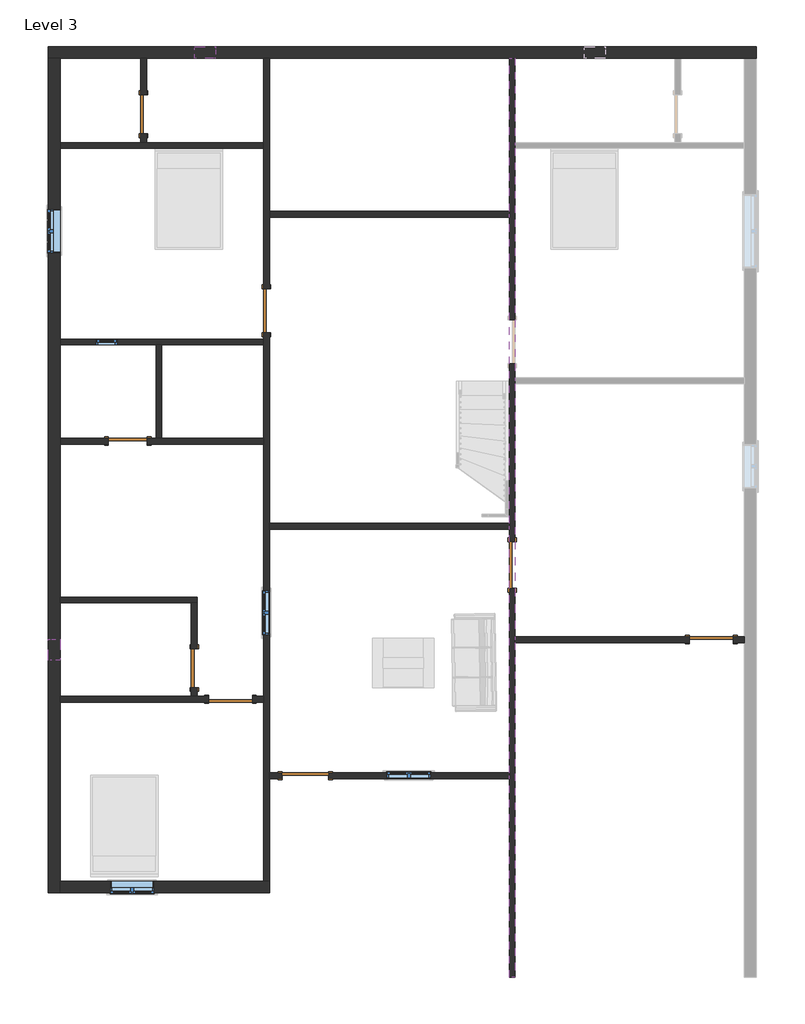
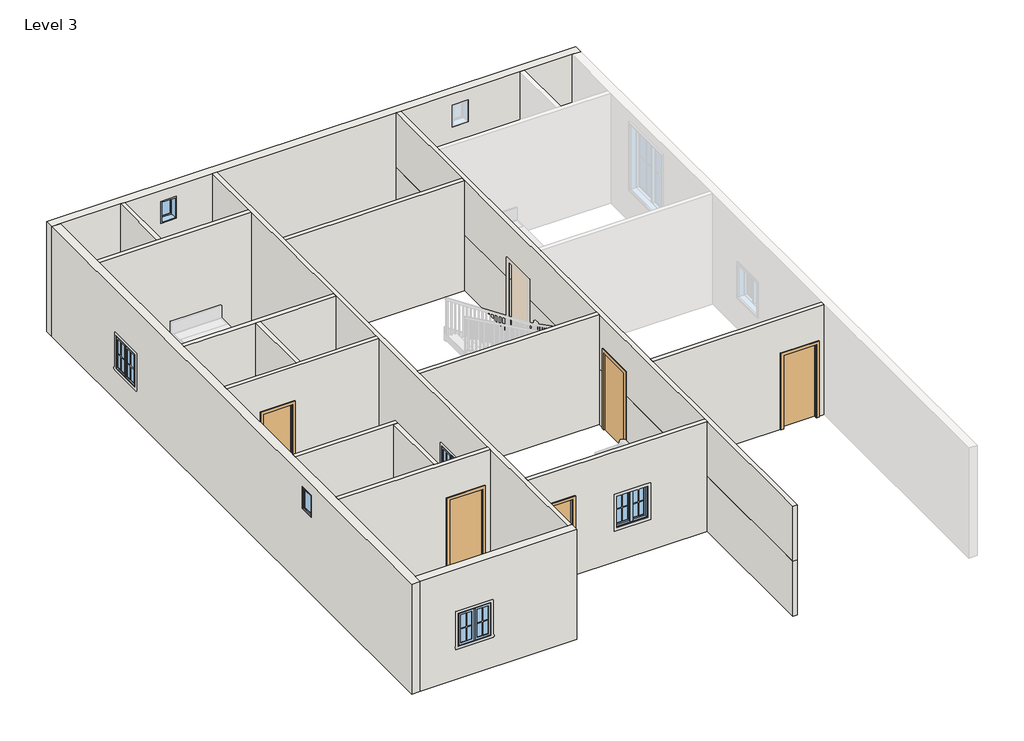
# One storey, part 1 of 3: 18 walls, 8 doors, 7 windows.
"""IFC4 building model written with IfcOpenShell, lengths in millimetres."""

from ifc_helpers import new_model, si_unit, frame, origin, place, context, project, spatial, polyline, outline, extrude, faceted_brep, transform, mapped, element, save
from components import door_f2b275c1, door_d8f5dbb5, door_825b8444, door_c29894e6, door_305aa2a5, window_aa618e30, window_a10b4202, window_339605e1, window_a598f463

model = new_model("IFC4")

# Units and contexts
model_context = context("Model", 3, world=origin())
ifc_project = project(units=[si_unit("LENGTHUNIT", "METRE", prefix="MILLI")], contexts=[model_context])

# Site, building, storey
site = spatial("IfcSite", under=ifc_project)
building = spatial("IfcBuilding", under=site)
storey = spatial("IfcBuildingStorey", under=building, Name="Level 3", Elevation=3200.4)

# Doors
placement = place(None, origin())
door_shape = door_f2b275c1(model_context)
element("IfcDoor", 1, ObjectType="Single-Flush : 30\" x 80\"", at=placement, inside=storey, context=model_context, shape_type="MappedRepresentation", body=[
    mapped(door_shape, transform((-5639.8561469, 9100.7522623, 3200.4), x_axis=(0.0, -1.0, 0.0), y_axis=(1.0, 0.0, 0.0), z_axis=(0.0, 0.0, 1.0))),
])
element("IfcDoor", 2, ObjectType="Single-Flush : 30\" x 80\"", at=placement, inside=storey, context=model_context, shape_type="MappedRepresentation", body=[
    mapped(door_shape, transform((-4646.033646, -1745.0477377, 3200.4), x_axis=(0.0, -1.0, 0.0), y_axis=(1.0, 0.0, 0.0), z_axis=(0.0, 0.0, 1.0))),
])
door_2_shape = door_d8f5dbb5(model_context)
element("IfcDoor", 3, ObjectType="Single-Flush : 30\" x 80\"", at=placement, inside=storey, context=model_context, shape_type="MappedRepresentation", body=[
    mapped(door_2_shape, transform((-5947.8915084, 2699.9522623, 3200.4), x_axis=(1.0, 0.0, 0.0), y_axis=(0.0, 1.0, 0.0), z_axis=(0.0, 0.0, 1.0))),
])
door_3_shape = door_825b8444(model_context)
element("IfcDoor", 4, ObjectType="Single-Flush : 34\" x 80\"", at=placement, inside=storey, context=model_context, shape_type="MappedRepresentation", body=[
    mapped(door_3_shape, transform((-3230.0915084, 5252.6522623, 3200.4), x_axis=(0.0, -1.0, 0.0), y_axis=(1.0, 0.0, 0.0), z_axis=(0.0, 0.0, 1.0))),
])
element("IfcDoor", 5, ObjectType="Single-Flush : 34\" x 80\"", at=placement, inside=storey, context=model_context, shape_type="MappedRepresentation", body=[
    mapped(door_3_shape, transform((-3938.0625772, -2354.6477377, 3200.4), x_axis=(1.0, 0.0, 0.0), y_axis=(0.0, 1.0, 0.0), z_axis=(0.0, 0.0, 1.0))),
])
door_4_shape = door_c29894e6(model_context)
element("IfcDoor", 6, ObjectType="Single-Flush : 34\" x 80\"", at=placement, inside=storey, context=model_context, shape_type="MappedRepresentation", body=[
    mapped(door_4_shape, transform((5488.4584916, -1186.2477377, 3200.4), x_axis=(1.0, 0.0, 0.0), y_axis=(0.0, 1.0, 0.0), z_axis=(0.0, 0.0, 1.0))),
])
door_5_shape = door_305aa2a5(model_context)
element("IfcDoor", 7, ObjectType="Single-Flush : 36\" x 84\"", at=placement, inside=storey, context=model_context, shape_type="MappedRepresentation", body=[
    mapped(door_5_shape, transform((1583.2084916, 274.2522623, 3200.4), x_axis=(0.0, -1.0, 0.0), y_axis=(1.0, 0.0, 0.0), z_axis=(0.0, 0.0, 1.0))),
])
element("IfcDoor", 8, ObjectType="Single-Flush : 36\" x 84\"", at=placement, inside=storey, context=model_context, shape_type="MappedRepresentation", body=[
    mapped(door_5_shape, transform((-2468.0915084, -3853.2477377, 3200.4), x_axis=(-1.0, 0.0, 0.0), y_axis=(0.0, -1.0, 0.0), z_axis=(0.0, 0.0, 1.0))),
])

# Walls
element("IfcWall", 9, ObjectType="9\"", at=placement, inside=storey, context=model_context, shape_type="Brep", body=[
    faceted_brep([(-7503.6415084, 10199.3022623, 3200.4), (-7275.0415084, 10199.3022623, 3200.4), (-5697.0061469, 10199.3022623, 3200.4), (-5582.7061469, 10199.3022623, 3200.4), (-3287.2415084, 10199.3022623, 3200.4), (-3172.9415084, 10199.3022623, 3200.4), (1526.0584916, 10199.3022623, 3200.4), (1640.3584916, 10199.3022623, 3200.4), (4770.1866507, 10199.3022623, 3200.4), (4884.4866507, 10199.3022623, 3200.4), (6136.1584916, 10199.3022623, 3200.4), (6364.7584916, 10199.3022623, 3200.4), (6364.7584916, 10199.3022623, 6248.4), (6136.1584916, 10199.3022623, 6248.4), (4884.4866507, 10199.3022623, 6248.4), (4770.1866507, 10199.3022623, 6248.4), (1640.3584916, 10199.3022623, 6248.4), (1526.0584916, 10199.3022623, 6248.4), (-3172.9415084, 10199.3022623, 6248.4), (-3287.2415084, 10199.3022623, 6248.4), (-5582.7061469, 10199.3022623, 6248.4), (-5697.0061469, 10199.3022623, 6248.4), (-7275.0415084, 10199.3022623, 6248.4), (-7503.6415084, 10199.3022623, 6248.4), (-4231.7738276, 10199.3022623, 5943.6), (-4231.7738276, 10199.3022623, 5334.0), (-4638.1738276, 10199.3022623, 5334.0), (-4638.1738276, 10199.3022623, 5943.6), (3408.4725711, 10199.3022623, 5943.6), (3408.4725711, 10199.3022623, 5334.0), (3002.0725711, 10199.3022623, 5334.0), (3002.0725711, 10199.3022623, 5943.6), (-7503.6415084, 10427.9022623, 3200.4), (-7503.6415084, 10427.9022623, 6248.4), (6364.7584916, 10427.9022623, 6248.4), (6364.7584916, 10427.9022623, 3200.4), (-4231.7738276, 10427.9022623, 5943.6), (-4638.1738276, 10427.9022623, 5943.6), (-4638.1738276, 10427.9022623, 5334.0), (-4231.7738276, 10427.9022623, 5334.0), (3408.4725711, 10427.9022623, 5943.6), (3002.0725711, 10427.9022623, 5943.6), (3002.0725711, 10427.9022623, 5334.0), (3408.4725711, 10427.9022623, 5334.0)], [[[0, 1, 2, 3, 4, 5, 6, 7, 8, 9, 10, 11, 12, 13, 14, 15, 16, 17, 18, 19, 20, 21, 22, 23], [24, 25, 26, 27], [28, 29, 30, 31]], [[32, 33, 34, 35], [36, 37, 38, 39], [40, 41, 42, 43]], [[11, 10, 9, 8, 7, 6, 5, 4, 3, 2, 1, 0, 32, 35]], [[0, 23, 33, 32]], [[12, 11, 35, 34]], [[25, 24, 36, 39]], [[26, 25, 39, 38]], [[27, 26, 38, 37]], [[24, 27, 37, 36]], [[29, 28, 40, 43]], [[30, 29, 43, 42]], [[31, 30, 42, 41]], [[28, 31, 41, 40]], [[23, 22, 21, 20, 19, 18, 17, 16, 15, 14, 13, 12, 34, 33]]]),
])
element("IfcWall", 10, ObjectType="9\"", at=placement, inside=storey, context=model_context, shape_type="Brep", body=[
    faceted_brep([(-7503.6415084, 10199.3022623, 3200.4), (-7503.6415084, -6145.5977377, 3200.4), (-7503.6415084, -6145.5977377, 6248.4), (-7503.6415084, 10199.3022623, 6248.4), (-7503.6415084, -1179.8977377, 5943.6), (-7503.6415084, -1586.2977377, 5943.6), (-7503.6415084, -1586.2977377, 5334.0), (-7503.6415084, -1179.8977377, 5334.0), (-7503.6415084, 7246.5522623, 5029.2), (-7503.6415084, 6382.9522623, 5029.2), (-7503.6415084, 6382.9522623, 4114.8), (-7503.6415084, 7246.5522623, 4114.8), (-7275.0415084, 10199.3022623, 3200.4), (-7275.0415084, 10199.3022623, 6248.4), (-7275.0415084, 8548.3022623, 6248.4), (-7275.0415084, 8434.0022623, 6248.4), (-7275.0415084, 4700.2022623, 6248.4), (-7275.0415084, 4585.9022623, 6248.4), (-7275.0415084, 2757.1022623, 6248.4), (-7275.0415084, 2642.8022623, 6248.4), (-7275.0415084, -354.3977377, 6248.4), (-7275.0415084, -468.6977377, 6248.4), (-7275.0415084, -2297.4977377, 6248.4), (-7275.0415084, -2411.7977377, 6248.4), (-7275.0415084, -5916.9977377, 6248.4), (-7275.0415084, -6145.5977377, 6248.4), (-7275.0415084, -6145.5977377, 3200.4), (-7275.0415084, -5916.9977377, 3200.4), (-7275.0415084, -2411.7977377, 3200.4), (-7275.0415084, -2297.4977377, 3200.4), (-7275.0415084, -468.6977377, 3200.4), (-7275.0415084, -354.3977377, 3200.4), (-7275.0415084, 2642.8022623, 3200.4), (-7275.0415084, 2757.1022623, 3200.4), (-7275.0415084, 4585.9022623, 3200.4), (-7275.0415084, 4700.2022623, 3200.4), (-7275.0415084, 8434.0022623, 3200.4), (-7275.0415084, 8548.3022623, 3200.4), (-7275.0415084, -1179.8977377, 5943.6), (-7275.0415084, -1179.8977377, 5334.0), (-7275.0415084, -1586.2977377, 5334.0), (-7275.0415084, -1586.2977377, 5943.6), (-7275.0415084, 7246.5522623, 5029.2), (-7275.0415084, 7246.5522623, 4114.8), (-7275.0415084, 6382.9522623, 4114.8), (-7275.0415084, 6382.9522623, 5029.2)], [[[0, 1, 2, 3], [4, 5, 6, 7], [8, 9, 10, 11]], [[12, 13, 14, 15, 16, 17, 18, 19, 20, 21, 22, 23, 24, 25, 26, 27, 28, 29, 30, 31, 32, 33, 34, 35, 36, 37], [38, 39, 40, 41], [42, 43, 44, 45]], [[1, 0, 12, 37, 36, 35, 34, 33, 32, 31, 30, 29, 28, 27, 26]], [[0, 3, 13, 12]], [[2, 1, 26, 25]], [[39, 38, 4, 7]], [[40, 39, 7, 6]], [[41, 40, 6, 5]], [[38, 41, 5, 4]], [[43, 42, 8, 11]], [[44, 43, 11, 10]], [[45, 44, 10, 9]], [[42, 45, 9, 8]], [[3, 2, 25, 24, 23, 22, 21, 20, 19, 18, 17, 16, 15, 14, 13]]]),
])
element("IfcWall", 11, ObjectType="9\"", at=placement, inside=storey, context=model_context, shape_type="Brep", body=[
    faceted_brep([(-7275.0415084, -6145.5977377, 3200.4), (-3172.9415084, -6145.5977377, 3200.4), (-3172.9415084, -6145.5977377, 6248.4), (-7275.0415084, -6145.5977377, 6248.4), (-6297.1415084, -6145.5977377, 5029.2), (-5433.5415084, -6145.5977377, 5029.2), (-5433.5415084, -6145.5977377, 4114.8), (-6297.1415084, -6145.5977377, 4114.8), (-7275.0415084, -5916.9977377, 3200.4), (-7275.0415084, -5916.9977377, 6248.4), (-3287.2415084, -5916.9977377, 6248.4), (-3172.9415084, -5916.9977377, 6248.4), (-3172.9415084, -5916.9977377, 3200.4), (-3287.2415084, -5916.9977377, 3200.4), (-6297.1415084, -5916.9977377, 5029.2), (-6297.1415084, -5916.9977377, 4114.8), (-5433.5415084, -5916.9977377, 4114.8), (-5433.5415084, -5916.9977377, 5029.2)], [[[0, 1, 2, 3], [4, 5, 6, 7]], [[8, 9, 10, 11, 12, 13], [14, 15, 16, 17]], [[1, 0, 8, 13, 12]], [[0, 3, 9, 8]], [[2, 1, 12, 11]], [[15, 14, 4, 7]], [[16, 15, 7, 6]], [[17, 16, 6, 5]], [[14, 17, 5, 4]], [[3, 2, 11, 10, 9]]]),
])
element("IfcWall", 12, ObjectType="WALL4.5\"", at=placement, inside=storey, context=model_context, shape_type="Brep", body=[
    faceted_brep([(-7275.0415084, 8434.0022623, 3200.4), (-3287.2415084, 8434.0022623, 3200.4), (-3287.2415084, 8434.0022623, 6248.4), (-7275.0415084, 8434.0022623, 6248.4), (-7275.0415084, 8548.3022623, 3200.4), (-7275.0415084, 8548.3022623, 6248.4), (-5697.0061469, 8548.3022623, 6248.4), (-5582.7061469, 8548.3022623, 6248.4), (-3287.2415084, 8548.3022623, 6248.4), (-3287.2415084, 8548.3022623, 3200.4), (-5582.7061469, 8548.3022623, 3200.4), (-5697.0061469, 8548.3022623, 3200.4)], [[[0, 1, 2, 3]], [[4, 5, 6, 7, 8, 9, 10, 11]], [[1, 0, 4, 11, 10, 9]], [[0, 3, 5, 4]], [[2, 1, 9, 8]], [[3, 2, 8, 7, 6, 5]]]),
])
element("IfcWall", 13, ObjectType="WALL4.5\"", at=placement, inside=storey, context=model_context, shape_type="SweptSolid", body=[
    extrude(outline(polyline([(8719.7522623, 5232.4), (8719.7522623, 3200.4), (8548.3022623, 3200.4), (8548.3022623, 6248.4), (10199.3022623, 6248.4), (10199.3022623, 3200.4), (9481.7522623, 3200.4), (9481.7522623, 5232.4), (8719.7522623, 5232.4)])), frame((-5697.0061469, 0.0, 0.0), z_axis=(1.0, 0.0, 0.0), x_axis=(0.0, 1.0, 0.0)), (0.0, 0.0, 1.0), 114.3),
])
element("IfcWall", 14, ObjectType="WALL4.5\"", at=placement, inside=storey, context=model_context, shape_type="Brep", body=[
    faceted_brep([(-3287.2415084, 4820.8522623, 5232.4), (-3287.2415084, 4820.8522623, 3200.4), (-3287.2415084, 4700.2022623, 3200.4), (-3287.2415084, 4585.9022623, 3200.4), (-3287.2415084, 2757.1022623, 3200.4), (-3287.2415084, 2642.8022623, 3200.4), (-3287.2415084, -2297.4977377, 3200.4), (-3287.2415084, -2411.7977377, 3200.4), (-3287.2415084, -5916.9977377, 3200.4), (-3287.2415084, -5916.9977377, 6248.4), (-3287.2415084, -2411.7977377, 6248.4), (-3287.2415084, -2297.4977377, 6248.4), (-3287.2415084, 2642.8022623, 6248.4), (-3287.2415084, 2757.1022623, 6248.4), (-3287.2415084, 4585.9022623, 6248.4), (-3287.2415084, 4700.2022623, 6248.4), (-3287.2415084, 8434.0022623, 6248.4), (-3287.2415084, 8548.3022623, 6248.4), (-3287.2415084, 10199.3022623, 6248.4), (-3287.2415084, 10199.3022623, 3200.4), (-3287.2415084, 8548.3022623, 3200.4), (-3287.2415084, 8434.0022623, 3200.4), (-3287.2415084, 5684.4522623, 3200.4), (-3287.2415084, 5684.4522623, 5232.4), (-3287.2415084, -227.3977377, 5029.2), (-3287.2415084, -1090.9977377, 5029.2), (-3287.2415084, -1090.9977377, 4114.8), (-3287.2415084, -227.3977377, 4114.8), (-3172.9415084, -5916.9977377, 3200.4), (-3172.9415084, -3910.3977377, 3200.4), (-3172.9415084, -3796.0977377, 3200.4), (-3172.9415084, 979.1022623, 3200.4), (-3172.9415084, 1093.4022623, 3200.4), (-3172.9415084, 4820.8522623, 3200.4), (-3172.9415084, 4820.8522623, 5232.4), (-3172.9415084, 5684.4522623, 5232.4), (-3172.9415084, 5684.4522623, 3200.4), (-3172.9415084, 7087.8022623, 3200.4), (-3172.9415084, 7202.1022623, 3200.4), (-3172.9415084, 10199.3022623, 3200.4), (-3172.9415084, 10199.3022623, 6248.4), (-3172.9415084, 7202.1022623, 6248.4), (-3172.9415084, 7087.8022623, 6248.4), (-3172.9415084, 1093.4022623, 6248.4), (-3172.9415084, 979.1022623, 6248.4), (-3172.9415084, -3796.0977377, 6248.4), (-3172.9415084, -3910.3977377, 6248.4), (-3172.9415084, -5916.9977377, 6248.4), (-3172.9415084, -227.3977377, 5029.2), (-3172.9415084, -227.3977377, 4114.8), (-3172.9415084, -1090.9977377, 4114.8), (-3172.9415084, -1090.9977377, 5029.2)], [[[0, 1, 2, 3, 4, 5, 6, 7, 8, 9, 10, 11, 12, 13, 14, 15, 16, 17, 18, 19, 20, 21, 22, 23], [24, 25, 26, 27]], [[28, 29, 30, 31, 32, 33, 34, 35, 36, 37, 38, 39, 40, 41, 42, 43, 44, 45, 46, 47], [48, 49, 50, 51]], [[22, 21, 20, 19, 39, 38, 37, 36]], [[8, 7, 6, 5, 4, 3, 2, 1, 33, 32, 31, 30, 29, 28]], [[9, 8, 28, 47]], [[19, 18, 40, 39]], [[34, 33, 1, 0]], [[35, 34, 0, 23]], [[36, 35, 23, 22]], [[49, 48, 24, 27]], [[50, 49, 27, 26]], [[51, 50, 26, 25]], [[48, 51, 25, 24]], [[18, 17, 16, 15, 14, 13, 12, 11, 10, 9, 47, 46, 45, 44, 43, 42, 41, 40]]]),
])
element("IfcWall", 15, ObjectType="WALL4.5\"", at=placement, inside=storey, context=model_context, shape_type="Brep", body=[
    faceted_brep([(-7275.0415084, 4585.9022623, 3200.4), (-5395.4415084, 4585.9022623, 3200.4), (-5281.1415084, 4585.9022623, 3200.4), (-3287.2415084, 4585.9022623, 3200.4), (-3287.2415084, 4585.9022623, 6248.4), (-5281.1415084, 4585.9022623, 6248.4), (-5395.4415084, 4585.9022623, 6248.4), (-7275.0415084, 4585.9022623, 6248.4), (-6160.6165084, 4585.9022623, 4724.4), (-6160.6165084, 4585.9022623, 4114.8), (-6567.0165084, 4585.9022623, 4114.8), (-6567.0165084, 4585.9022623, 4724.4), (-7275.0415084, 4700.2022623, 3200.4), (-7275.0415084, 4700.2022623, 6248.4), (-3287.2415084, 4700.2022623, 6248.4), (-3287.2415084, 4700.2022623, 3200.4), (-6160.6165084, 4700.2022623, 4724.4), (-6567.0165084, 4700.2022623, 4724.4), (-6567.0165084, 4700.2022623, 4114.8), (-6160.6165084, 4700.2022623, 4114.8)], [[[0, 1, 2, 3, 4, 5, 6, 7], [8, 9, 10, 11]], [[12, 13, 14, 15], [16, 17, 18, 19]], [[3, 2, 1, 0, 12, 15]], [[0, 7, 13, 12]], [[4, 3, 15, 14]], [[9, 8, 16, 19]], [[10, 9, 19, 18]], [[11, 10, 18, 17]], [[8, 11, 17, 16]], [[7, 6, 5, 4, 14, 13]]]),
])
element("IfcWall", 16, ObjectType="WALL4.5\"", at=placement, inside=storey, context=model_context, shape_type="SweptSolid", body=[
    extrude(outline(polyline([(-5395.4415084, 2757.1022623), (-5395.4415084, 4585.9022623), (-5281.1415084, 4585.9022623), (-5281.1415084, 2757.1022623), (-5395.4415084, 2757.1022623)])), frame((0.0, 0.0, 3200.4), z_axis=(0.0, 0.0, 1.0), x_axis=(1.0, 0.0, 0.0)), (0.0, 0.0, 1.0), 3048.0),
])
element("IfcWall", 17, ObjectType="WALL4.5\"", at=placement, inside=storey, context=model_context, shape_type="Brep", body=[
    faceted_brep([(-5566.8915084, 2642.8022623, 5232.4), (-5566.8915084, 2642.8022623, 3200.4), (-3287.2415084, 2642.8022623, 3200.4), (-3287.2415084, 2642.8022623, 6248.4), (-7275.0415084, 2642.8022623, 6248.4), (-7275.0415084, 2642.8022623, 3200.4), (-6328.8915084, 2642.8022623, 3200.4), (-6328.8915084, 2642.8022623, 5232.4), (-3287.2415084, 2757.1022623, 3200.4), (-5281.1415084, 2757.1022623, 3200.4), (-5395.4415084, 2757.1022623, 3200.4), (-5566.8915084, 2757.1022623, 3200.4), (-5566.8915084, 2757.1022623, 5232.4), (-6328.8915084, 2757.1022623, 5232.4), (-6328.8915084, 2757.1022623, 3200.4), (-7275.0415084, 2757.1022623, 3200.4), (-7275.0415084, 2757.1022623, 6248.4), (-5395.4415084, 2757.1022623, 6248.4), (-5281.1415084, 2757.1022623, 6248.4), (-3287.2415084, 2757.1022623, 6248.4)], [[[0, 1, 2, 3, 4, 5, 6, 7]], [[8, 9, 10, 11, 12, 13, 14, 15, 16, 17, 18, 19]], [[6, 5, 15, 14]], [[2, 1, 11, 10, 9, 8]], [[5, 4, 16, 15]], [[3, 2, 8, 19]], [[12, 11, 1, 0]], [[13, 12, 0, 7]], [[14, 13, 7, 6]], [[4, 3, 19, 18, 17, 16]]]),
])
element("IfcWall", 18, ObjectType="WALL4.5\"", at=placement, inside=storey, context=model_context, shape_type="Brep", body=[
    faceted_brep([(-7275.0415084, -468.6977377, 3200.4), (-4703.183646, -468.6977377, 3200.4), (-4588.883646, -468.6977377, 3200.4), (-4588.883646, -468.6977377, 6248.4), (-4703.183646, -468.6977377, 6248.4), (-7275.0415084, -468.6977377, 6248.4), (-7275.0415084, -354.3977377, 3200.4), (-7275.0415084, -354.3977377, 6248.4), (-4588.883646, -354.3977377, 6248.4), (-4588.883646, -354.3977377, 3200.4)], [[[0, 1, 2, 3, 4, 5]], [[6, 7, 8, 9]], [[2, 1, 0, 6, 9]], [[0, 5, 7, 6]], [[3, 2, 9, 8]], [[5, 4, 3, 8, 7]]]),
])
element("IfcWall", 19, ObjectType="WALL4.5\"", at=placement, inside=storey, context=model_context, shape_type="SweptSolid", body=[
    extrude(outline(polyline([(-2126.0477377, 5232.4), (-2126.0477377, 3200.4), (-2297.4977377, 3200.4), (-2297.4977377, 6248.4), (-468.6977377, 6248.4), (-468.6977377, 3200.4), (-1364.0477377, 3200.4), (-1364.0477377, 5232.4), (-2126.0477377, 5232.4)])), frame((-4703.183646, 0.0, 0.0), z_axis=(1.0, 0.0, 0.0), x_axis=(0.0, 1.0, 0.0)), (0.0, 0.0, 1.0), 114.3),
])
element("IfcWall", 20, ObjectType="WALL4.5\"", at=placement, inside=storey, context=model_context, shape_type="Brep", body=[
    faceted_brep([(-3506.2625772, -2411.7977377, 5232.4), (-3506.2625772, -2411.7977377, 3200.4), (-3287.2415084, -2411.7977377, 3200.4), (-3287.2415084, -2411.7977377, 6248.4), (-7275.0415084, -2411.7977377, 6248.4), (-7275.0415084, -2411.7977377, 3200.4), (-4369.8625772, -2411.7977377, 3200.4), (-4369.8625772, -2411.7977377, 5232.4), (-3287.2415084, -2297.4977377, 3200.4), (-3506.2625772, -2297.4977377, 3200.4), (-3506.2625772, -2297.4977377, 5232.4), (-4369.8625772, -2297.4977377, 5232.4), (-4369.8625772, -2297.4977377, 3200.4), (-4588.883646, -2297.4977377, 3200.4), (-4703.183646, -2297.4977377, 3200.4), (-7275.0415084, -2297.4977377, 3200.4), (-7275.0415084, -2297.4977377, 6248.4), (-4703.183646, -2297.4977377, 6248.4), (-4588.883646, -2297.4977377, 6248.4), (-3287.2415084, -2297.4977377, 6248.4)], [[[0, 1, 2, 3, 4, 5, 6, 7]], [[8, 9, 10, 11, 12, 13, 14, 15, 16, 17, 18, 19]], [[6, 5, 15, 14, 13, 12]], [[2, 1, 9, 8]], [[5, 4, 16, 15]], [[3, 2, 8, 19]], [[10, 9, 1, 0]], [[11, 10, 0, 7]], [[12, 11, 7, 6]], [[4, 3, 19, 18, 17, 16]]]),
])
element("IfcWall", 21, ObjectType="WALL4.5\"", at=placement, inside=storey, context=model_context, shape_type="SweptSolid", body=[
    extrude(outline(polyline([(1526.0584916, 7087.8022623), (-3172.9415084, 7087.8022623), (-3172.9415084, 7202.1022623), (1526.0584916, 7202.1022623), (1526.0584916, 7087.8022623)])), frame((0.0, 0.0, 3200.4), z_axis=(0.0, 0.0, 1.0), x_axis=(1.0, 0.0, 0.0)), (0.0, 0.0, 1.0), 3048.0),
])
element("IfcWall", 22, ObjectType="WALL4.5\"", at=placement, inside=storey, context=model_context, shape_type="Brep", body=[
    faceted_brep([(1526.0584916, -7802.9477377, 3200.4), (1526.0584916, -7802.9477377, 4724.4), (1526.0584916, -182.9477377, 4724.4), (1526.0584916, -182.9477377, 3200.4), (1526.0584916, -3796.0977377, 3200.4), (1526.0584916, -3910.3977377, 3200.4), (1640.3584916, -7802.9477377, 4724.4), (1640.3584916, -7802.9477377, 3200.4), (1640.3584916, -1243.3977377, 3200.4), (1640.3584916, -1129.0977377, 3200.4), (1640.3584916, -182.9477377, 3200.4), (1640.3584916, -182.9477377, 4724.4)], [[[0, 1, 2, 3, 4, 5]], [[6, 7, 8, 9, 10, 11]], [[7, 0, 5, 4, 3, 10, 9, 8]], [[1, 0, 7, 6]], [[1, 6, 11, 2]], [[3, 2, 11, 10]]]),
    faceted_brep([(1526.0584916, 10199.3022623, 4724.4), (1526.0584916, 10199.3022623, 3200.4), (1526.0584916, 7202.1022623, 3200.4), (1526.0584916, 7087.8022623, 3200.4), (1526.0584916, 5074.8522623, 3200.4), (1526.0584916, 5074.8522623, 4724.4), (1640.3584916, 10199.3022623, 3200.4), (1640.3584916, 10199.3022623, 4724.4), (1640.3584916, 5074.8522623, 4724.4), (1640.3584916, 5074.8522623, 3200.4), (1640.3584916, 8434.0022623, 3200.4), (1640.3584916, 8548.3022623, 3200.4)], [[[0, 1, 2, 3, 4, 5]], [[6, 7, 8, 9, 10, 11]], [[1, 6, 11, 10, 9, 4, 3, 2]], [[7, 0, 5, 8]], [[1, 0, 7, 6]], [[5, 4, 9, 8]]]),
    faceted_brep([(1526.0584916, 4211.2522623, 4724.4), (1526.0584916, 4211.2522623, 3200.4), (1526.0584916, 1093.4022623, 3200.4), (1526.0584916, 979.1022623, 3200.4), (1526.0584916, 731.4522623, 3200.4), (1526.0584916, 731.4522623, 4724.4), (1640.3584916, 4211.2522623, 3200.4), (1640.3584916, 4211.2522623, 4724.4), (1640.3584916, 731.4522623, 4724.4), (1640.3584916, 731.4522623, 3200.4), (1640.3584916, 3823.9022623, 3200.4), (1640.3584916, 3938.2022623, 3200.4)], [[[0, 1, 2, 3, 4, 5]], [[6, 7, 8, 9, 10, 11]], [[1, 6, 11, 10, 9, 4, 3, 2]], [[7, 0, 5, 8]], [[1, 0, 7, 6]], [[5, 4, 9, 8]]]),
])
element("IfcWall", 23, ObjectType="WALL4.5\"", at=placement, inside=storey, context=model_context, shape_type="SweptSolid", body=[
    extrude(outline(polyline([(3200.4, -3172.9415084), (3200.4, -2925.2915084), (5334.0, -2925.2915084), (5334.0, -2010.8915084), (3200.4, -2010.8915084), (3200.4, 1526.0584916), (6248.4, 1526.0584916), (6248.4, -3172.9415084), (3200.4, -3172.9415084)]), holes=[polyline([(5029.2, -10.6415084), (4114.8, -10.6415084), (4114.8, -874.2415084), (5029.2, -874.2415084), (5029.2, -10.6415084)])]), frame((0.0, -3910.3977377, 0.0), z_axis=(0.0, 1.0, 0.0), x_axis=(0.0, 0.0, 1.0)), (0.0, 0.0, 1.0), 114.3),
])
element("IfcWall", 24, ObjectType="WALL4.5\"", at=placement, inside=storey, context=model_context, shape_type="SweptSolid", body=[
    extrude(outline(polyline([(1526.0584916, 979.1022623), (-3172.9415084, 979.1022623), (-3172.9415084, 1093.4022623), (1526.0584916, 1093.4022623), (1526.0584916, 979.1022623)])), frame((0.0, 0.0, 3200.4), z_axis=(0.0, 0.0, 1.0), x_axis=(1.0, 0.0, 0.0)), (0.0, 0.0, 1.0), 3048.0),
])
element("IfcWall", 25, ObjectType="WALL4.5\"", at=placement, inside=storey, context=model_context, shape_type="SweptSolid", body=[
    extrude(outline(polyline([(5232.4, 5920.2584916), (3200.4, 5920.2584916), (3200.4, 6136.1584916), (6248.4, 6136.1584916), (6248.4, 1640.3584916), (3200.4, 1640.3584916), (3200.4, 5056.6584916), (5232.4, 5056.6584916), (5232.4, 5920.2584916)])), frame((0.0, -1243.3977377, 0.0), z_axis=(0.0, 1.0, 0.0), x_axis=(0.0, 0.0, 1.0)), (0.0, 0.0, 1.0), 114.3),
])
element("IfcWall", 26, ObjectType="WALL4.5\"", at=placement, inside=storey, context=model_context, shape_type="Brep", body=[
    faceted_brep([(1526.0584916, -7802.9477377, 4724.4), (1526.0584916, -7802.9477377, 6248.4), (1526.0584916, -3910.3977377, 6248.4), (1526.0584916, -3796.0977377, 6248.4), (1526.0584916, 979.1022623, 6248.4), (1526.0584916, 1093.4022623, 6248.4), (1526.0584916, 7087.8022623, 6248.4), (1526.0584916, 7202.1022623, 6248.4), (1526.0584916, 10199.3022623, 6248.4), (1526.0584916, 10199.3022623, 4724.4), (1526.0584916, 5074.8522623, 4724.4), (1526.0584916, 5074.8522623, 5232.4), (1526.0584916, 4211.2522623, 5232.4), (1526.0584916, 4211.2522623, 4724.4), (1526.0584916, 731.4522623, 4724.4), (1526.0584916, 731.4522623, 5334.0), (1526.0584916, -182.9477377, 5334.0), (1526.0584916, -182.9477377, 4724.4), (1640.3584916, -7802.9477377, 6248.4), (1640.3584916, -7802.9477377, 4724.4), (1640.3584916, -182.9477377, 4724.4), (1640.3584916, -182.9477377, 5334.0), (1640.3584916, 731.4522623, 5334.0), (1640.3584916, 731.4522623, 4724.4), (1640.3584916, 4211.2522623, 4724.4), (1640.3584916, 4211.2522623, 5232.4), (1640.3584916, 5074.8522623, 5232.4), (1640.3584916, 5074.8522623, 4724.4), (1640.3584916, 10199.3022623, 4724.4), (1640.3584916, 10199.3022623, 6248.4), (1640.3584916, 8548.3022623, 6248.4), (1640.3584916, 8434.0022623, 6248.4), (1640.3584916, 3938.2022623, 6248.4), (1640.3584916, 3823.9022623, 6248.4), (1640.3584916, -1129.0977377, 6248.4), (1640.3584916, -1243.3977377, 6248.4)], [[[0, 1, 2, 3, 4, 5, 6, 7, 8, 9, 10, 11, 12, 13, 14, 15, 16, 17]], [[18, 19, 20, 21, 22, 23, 24, 25, 26, 27, 28, 29, 30, 31, 32, 33, 34, 35]], [[19, 0, 17, 20]], [[13, 24, 23, 14]], [[10, 9, 28, 27]], [[1, 0, 19, 18]], [[12, 25, 24, 13]], [[25, 12, 11, 26]], [[26, 11, 10, 27]], [[16, 21, 20, 17]], [[21, 16, 15, 22]], [[22, 15, 14, 23]], [[9, 8, 29, 28]], [[8, 7, 6, 5, 4, 3, 2, 1, 18, 35, 34, 33, 32, 31, 30, 29]]]),
])

# Windows
window_shape = window_aa618e30(model_context)
element("IfcWindow", 27, ObjectType="Fixed : 16\" x 24\"", at=placement, inside=storey, context=model_context, shape_type="MappedRepresentation", body=[
    mapped(window_shape, transform((-4396.8738276, 10313.6022623, 4419.6), x_axis=(1.0, 0.0, 0.0), y_axis=(0.0, 1.0, 0.0), z_axis=(0.0, 0.0, 1.0))),
])
element("IfcWindow", 28, ObjectType="Fixed : 16\" x 24\"", at=placement, inside=storey, context=model_context, shape_type="MappedRepresentation", body=[
    mapped(window_shape, transform((-7389.3415084, -1344.9977377, 4419.6), x_axis=(0.0, 1.0, 0.0), y_axis=(-1.0, 0.0, 0.0), z_axis=(0.0, 0.0, 1.0))),
])
window_2_shape = window_a10b4202(model_context)
element("IfcWindow", 29, ObjectType="Fixed : 16\" x 24\"", at=placement, inside=storey, context=model_context, shape_type="MappedRepresentation", body=[
    mapped(window_2_shape, transform((-6325.7165084, 4643.0522623, 3200.4), x_axis=(1.0, 0.0, 0.0), y_axis=(0.0, 1.0, 0.0), z_axis=(0.0, 0.0, 1.0))),
])
window_3_shape = window_339605e1(model_context)
element("IfcWindow", 30, ObjectType="Window-Casement-Double : 34\" x 36\"", at=placement, inside=storey, context=model_context, shape_type="MappedRepresentation", body=[
    mapped(window_3_shape, transform((-7389.3415084, 6814.7522623, 3200.4), x_axis=(0.0, 1.0, 0.0), y_axis=(-1.0, 0.0, 0.0), z_axis=(0.0, 0.0, 1.0))),
])
element("IfcWindow", 31, ObjectType="Window-Casement-Double : 34\" x 36\"", at=placement, inside=storey, context=model_context, shape_type="MappedRepresentation", body=[
    mapped(window_3_shape, transform((-5865.3415084, -6031.2977377, 3200.4), x_axis=(-1.0, 0.0, 0.0), y_axis=(0.0, -1.0, 0.0), z_axis=(0.0, 0.0, 1.0))),
])
window_4_shape = window_a598f463(model_context)
element("IfcWindow", 32, ObjectType="Window-Casement-Double : 34\" x 36\"", at=placement, inside=storey, context=model_context, shape_type="MappedRepresentation", body=[
    mapped(window_4_shape, transform((-442.4415084, -3853.2477377, 3200.4), x_axis=(1.0, 0.0, 0.0), y_axis=(0.0, 1.0, 0.0), z_axis=(0.0, 0.0, 1.0))),
])
element("IfcWindow", 33, ObjectType="Window-Casement-Double : 34\" x 36\"", at=placement, inside=storey, context=model_context, shape_type="MappedRepresentation", body=[
    mapped(window_4_shape, transform((-3230.0915084, -659.1977377, 3200.4), x_axis=(0.0, 1.0, 0.0), y_axis=(-1.0, 0.0, 0.0), z_axis=(0.0, 0.0, 1.0))),
])

save(model, "model.ifc")

# Revit data of these elements
# Type "Single-Flush : 30\" x 80\""
#   Type Mark = "5"
#   Construction Type Id = "MDOOR"
#   Assembly Code = "C1020"
#   Analytic Construction = "Metal"
#   Thickness = 0' - 2"
#   Heat Transfer Coefficient (U) = 0.651978 BTU/(h·ft²·°F)
#   Height = 6' - 8"
#   Trim Projection Ext = 0' - 1"
#   Trim Projection Int = 0' - 1"
#   Trim Width = 0' - 3"
#   Width = 2' - 6"
#   Define Thermal Properties by = 1
#   Define Thermal Properties by = 1
#   Door Material = Door - Panel
#   Frame Material = Door - Frame
#   Visual Light Transmittance = 0
#   Solar Heat Gain Coefficient = 0
#   Function = (empty or 0)
#   Wall Closure = (empty or 0)
# Type "Single-Flush : 34\" x 80\""
#   Type Mark = "7"
#   Construction Type Id = "MDOOR"
#   Assembly Code = "C1020"
#   Analytic Construction = "Metal"
#   Thickness = 0' - 2"
#   Heat Transfer Coefficient (U) = 0.651978 BTU/(h·ft²·°F)
#   Height = 6' - 8"
#   Trim Projection Ext = 0' - 1"
#   Trim Projection Int = 0' - 1"
#   Trim Width = 0' - 3"
#   Width = 2' - 10"
#   Define Thermal Properties by = 1
#   Define Thermal Properties by = 1
#   Door Material = Door - Panel
#   Frame Material = Door - Frame
#   Visual Light Transmittance = 0
#   Solar Heat Gain Coefficient = 0
#   Function = (empty or 0)
#   Wall Closure = (empty or 0)
# Type "Single-Flush : 36\" x 84\""
#   Type Mark = "1"
#   Construction Type Id = "MDOOR"
#   Assembly Code = "C1020"
#   Analytic Construction = "Metal"
#   Thickness = 0' - 2"
#   Heat Transfer Coefficient (U) = 0.651978 BTU/(h·ft²·°F)
#   Height = 7' - 0"
#   Trim Projection Ext = 0' - 1"
#   Trim Projection Int = 0' - 1"
#   Trim Width = 0' - 3"
#   Width = 3' - 0"
#   Define Thermal Properties by = 1
#   Define Thermal Properties by = 1
#   Door Material = Door - Panel
#   Frame Material = Door - Frame
#   Visual Light Transmittance = 0
#   Solar Heat Gain Coefficient = 0
#   Function = (empty or 0)
#   Wall Closure = (empty or 0)
# Type "9\""
#   Assembly Code = "B2010"
#   Layers, outside or top first: 0' - 9" no material (function 1)
# Type "WALL4.5\""
#   Assembly Code = "B2010"
#   Layers, outside or top first: 0' - 4 1/2" no material (function 1)
# Type "Fixed : 16\" x 24\""
#   Type Mark = "4"
#   Construction Type Id = "GSP4R"
#   Assembly Code = "B2020100"
#   Analytic Construction = "1/8 in Pilkington single glazing"
#   Visual Light Transmittance = 0.9
#   Solar Heat Gain Coefficient = 0.78
#   Heat Transfer Coefficient (U) = 0.6496 BTU/(h·ft²·°F)
#   Height = 2' - 0"
#   Default Sill Height = 3' - 0"
#   Width = 1' - 4"
#   Window Inset = 0' - 0 3/4"
#   Define Thermal Properties by = 1
#   Define Thermal Properties by = 1
#   Glass Pane Material = Glass
#   Sash Material = Sash
#   Wall Closure = (empty or 0)
# Type "Window-Casement-Double : 34\" x 36\""
#   Type Mark = "14"
#   Fire Rating = "0.5h"
#   Assembly Code = "B2020100"
#   Analytic Construction = "Double glazing - domestic"
#   Frame Extension [instance default] = 0' - 0 1/4"
#   Window Inset [instance default] = 0' - 0"
#   Wall Thickness [instance default] = 0' - 6"
#   Interior Wall Closure [instance default] = 0' - 2 1/4"
#   Half Width = 1' - 5"
#   Visual Light Transmittance = 0.81
#   Thermal Resistance (R) = 1.8146 (h·ft²·°F)/BTU
#   Solar Heat Gain Coefficient = 0.76
#   Rough Width = 2' - 10 1/2"
#   Rough Height = 3' - 0 1/2"
#   Height = 3' - 0"
#   Heat Transfer Coefficient (U) = 0.5511 BTU/(h·ft²·°F)
#   Exterior Wall Closure [instance default] = 0' - 1 1/4"
#   Extension Jamb [instance default] = 0' - 2 1/4"
#   Default Sill Height = 3' - 0"
#   Width = 2' - 10"
#   Define Thermal Properties by = 0
#   Muntin Visibility = yes
#   Interior Trim Visibility [instance default] = yes
#   Exterior Trim Visibility [instance default] = yes
#   Extension Jamb Visibility [instance default] = yes
#   Interior Trim Material = Wood - Stained
#   Muntin Pattern = Muntin Pattern_2x2 : Muntin Pattern_2x2
#   Interior Trim = Trim-Window-Interior-Flat : Picture Frame
#   Interior Frame Material = Wood - Stained
#   Glass Panel Material = Glass
#   Exterior Trim Material = Clad - White
#   Exterior Trim = Trim-Window-Exterior-Flat : with Sill
#   Exterior Frame Material = Clad - White
#   Wall Closure = (empty or 0)
# Elements 1, 2, 3 (IfcDoor, "Single-Flush : 30\" x 80\"")
#   Phase Created = New Construction
#   Materials on its faces: "Door - Frame", "Door - Panel"
# Elements 4, 5, 6 (IfcDoor, "Single-Flush : 34\" x 80\"")
#   Phase Created = New Construction
#   Materials on its faces: "Door - Frame", "Door - Panel"
# Elements 7, 8 (IfcDoor, "Single-Flush : 36\" x 84\"")
#   Phase Created = New Construction
#   Materials on its faces: "Door - Frame", "Door - Panel"
# Elements 9, 10, 11 (IfcWall, "9\"")
#   Top Offset = 0' - 0"
#   Base Offset = 0' - 0"
#   Unconnected Height = 10' - 0"
#   wall height = 10' - 0"
#   Phase Created = New Construction
#   Base Constraint = Level 3
#   Materials on its faces: "Default Wall", "legs"
# Elements 12, 13, 15, 16, 17, 18, 19, 20, 21, 24 (IfcWall, "WALL4.5\"")
#   Top Offset = 0' - 0"
#   Base Offset = 0' - 0"
#   Unconnected Height = 10' - 0"
#   wall height = 10' - 0"
#   Phase Created = New Construction
#   Base Constraint = Level 3
#   Materials on its faces: "Default Wall"
# Elements 14, 23, 25 (IfcWall, "WALL4.5\"")
#   Top Offset = 0' - 0"
#   Base Offset = 0' - 0"
#   Unconnected Height = 10' - 0"
#   wall height = 10' - 0"
#   Phase Created = New Construction
#   Base Constraint = Level 3
#   Materials on its faces: "Default Wall", "legs"
# Element 22 (IfcWall, "WALL4.5\"")
#   Top Offset = 0' - 0"
#   Base Offset = 0' - 0"
#   Unconnected Height = 5' - 0"
#   wall height = 5' - 0"
#   Phase Created = New Construction
#   Base Constraint = Level 3
#   Materials on its faces: "Default Wall", "legs"
# Element 26 (IfcWall, "WALL4.5\"")
#   built-in parameter 1001111 = 5' - 0"
#   Top Offset = 0' - 0"
#   Base Offset = 5' - 0"
#   Unconnected Height = 5' - 0"
#   wall height = 5' - 0"
#   Phase Created = New Construction
#   Base Constraint = Level 3
#   Materials on its faces: "Default Wall", "legs", "Cherry"
# Element 27 (IfcWindow, "Fixed : 16\" x 24\"")
#   Mark = "11"
#   Phase Created = New Construction
#   Materials on its faces: "Sash", "Glass"
# Element 28 (IfcWindow, "Fixed : 16\" x 24\"")
#   Mark = "14"
#   Phase Created = New Construction
#   Materials on its faces: "Sash", "Glass"
# Element 29 (IfcWindow, "Fixed : 16\" x 24\"")
#   Mark = "13"
#   Phase Created = New Construction
#   Materials on its faces: "Sash", "Glass"
# Element 30 (IfcWindow, "Window-Casement-Double : 34\" x 36\"")
#   Mark = "15"
#   Window Inset = 0' - 0"
#   Interior Wall Closure = 0' - 2 1/4"
#   Frame Extension = 0' - 0 1/4"
#   Exterior Wall Closure = 0' - 1 1/4"
#   Interior Trim Visibility = yes
#   Exterior Trim Visibility = yes
#   Phase Created = New Construction
#   Materials on its faces: "Wood - Stained", "Glass", "Clad - White"
# Element 31 (IfcWindow, "Window-Casement-Double : 34\" x 36\"")
#   Mark = "16"
#   Window Inset = 0' - 0"
#   Interior Wall Closure = 0' - 2 1/4"
#   Frame Extension = 0' - 0 1/4"
#   Exterior Wall Closure = 0' - 1 1/4"
#   Interior Trim Visibility = yes
#   Exterior Trim Visibility = yes
#   Phase Created = New Construction
#   Materials on its faces: "Wood - Stained", "Glass", "Clad - White"
# Element 32 (IfcWindow, "Window-Casement-Double : 34\" x 36\"")
#   Mark = "17"
#   Window Inset = 0' - 0"
#   Interior Wall Closure = 0' - 2 1/4"
#   Frame Extension = 0' - 0 1/4"
#   Exterior Wall Closure = 0' - 1 1/4"
#   Interior Trim Visibility = yes
#   Exterior Trim Visibility = yes
#   Phase Created = New Construction
#   Materials on its faces: "Wood - Stained", "Glass", "Clad - White"
# Element 33 (IfcWindow, "Window-Casement-Double : 34\" x 36\"")
#   Mark = "20"
#   Window Inset = 0' - 0"
#   Interior Wall Closure = 0' - 2 1/4"
#   Frame Extension = 0' - 0 1/4"
#   Exterior Wall Closure = 0' - 1 1/4"
#   Interior Trim Visibility = yes
#   Exterior Trim Visibility = yes
#   Phase Created = New Construction
#   Materials on its faces: "Wood - Stained", "Glass", "Clad - White"
# Materials
#   "Door - Panel": class "Wood", colour RGB 210 159 95, transparency 0, Cost = 0
#   "Door - Frame": colour RGB 118 70 51, transparency 0, Cost = 0
#   "Glass": class "Glass", colour RGB 0 128 192, transparency 0.75, Description = "Soda Lime Glass", Cost = 0
#   "Sash": class "Wood", colour RGB 224 178 126, transparency 0, Cost = 0
#   "Wood - Stained": class "Wood", colour RGB 224 178 126, transparency 0, Cost = 0
#   "Clad - White": class "Wood", colour RGB 242 242 238, transparency 0, Cost = 0
#   "Default Wall": colour RGB 128 128 128, transparency 0, Cost = 0
#   "legs": colour RGB 90 73 37, transparency 0, Cost = 0
#   "Cherry": class "Wood", colour RGB 226 177 128, transparency 0, Description = "Prunus Serotina", Cost = 0
